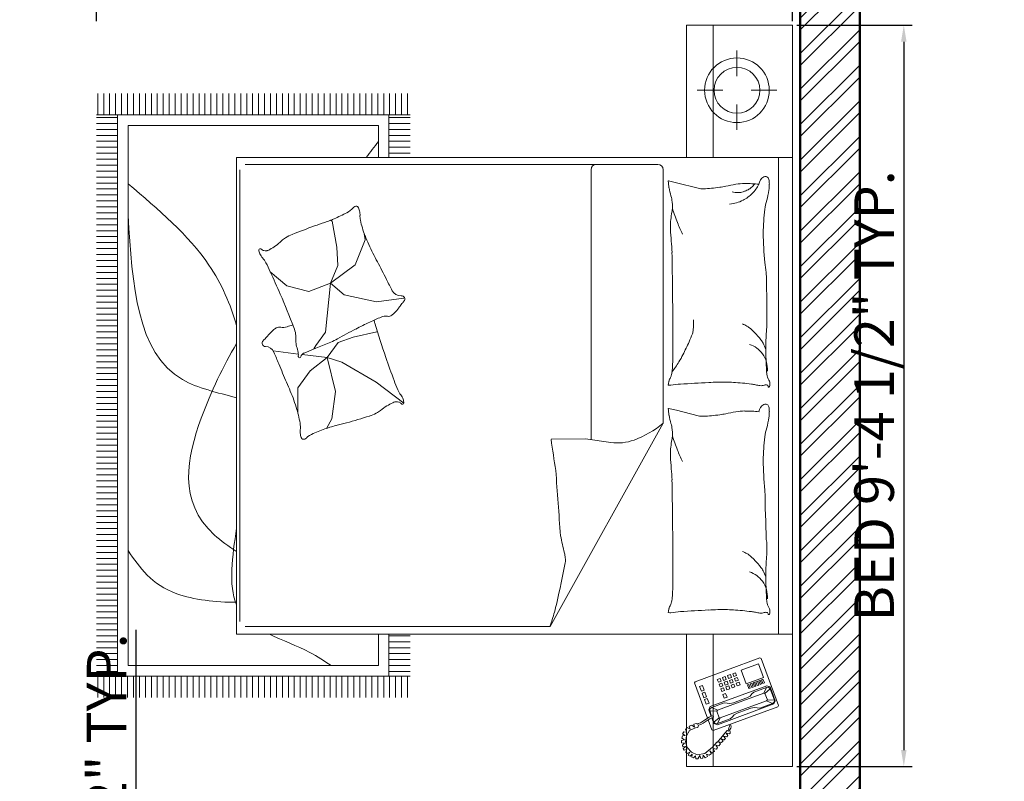
# Model space of a CAD drawing. Units: millimetres. Extents: x 20768 to 23556, y 50760 to 52704.
# Tile 22 of 36: x 21006 to 21155, y 52368 to 52483. Entities that reach past the tile are written whole.
import ezdxf

# ---------------------------------------------------------------- set-up
doc = ezdxf.new("R2010")
doc.units = ezdxf.units.MM
for name, color, linetype, lineweight in [('A-FURN', 8, 'Continuous', 18), ('A-WALL', 7, 'Continuous', 50), ('A-WALL-PATT', 8, 'Continuous', 13), ('S-ANNO-DIMS', 2, 'Continuous', 18)]:
    doc.layers.add(name, color=color, linetype=linetype, lineweight=lineweight)
doc.styles.add('DIM_FONT', font='SIMPLEX.shx', dxfattribs={"width": 0.8})
doc.styles.get("Standard").update_dxf_attribs({"font": 'arial.ttf'})
doc.dimstyles.new('ISO-25', dxfattribs={"dimtxt": 6, "dimasz": 2.5, "dimexe": 1.25, "dimexo": 0.625, "dimtad": 1, "dimdec": 0, "dimlunit": 3, "dimtxsty": 'Standard', "dimcen": 2.5, "dimadec": 0, "dimazin": 0, "dimtfac": 1, "dimtdec": 0, "dimtmove": 0, "dimatfit": 3, "dimfxl": 1, "dimarcsym": 0})

# ---------------------------------------------------------------- blocks, each defined once
blk = doc.blocks.new('A$C4F634EDD')
for p, q in [((0, 2.6295), (0, 2.2295)), ((0.5, 2.6295), (0, 2.6295)), ((0.5, 2.6295), (2.3, 2.6295)), ((0.5, 0.5295), (0.5, 2.6295)), ((0.5, 2.2295), (0.5, 2.6295)), ((2.3, 2.6295), (2.3, 0.5295)), ((2.3, 2.6295), (2.8, 2.6295)), ((2.3, 2.2295), (2.3, 2.6295)), ((2.8, 2.6295), (2.8, 2.2295)), ((0.2457, 2.5697), (0.2457, 2.4733)), ((0.5, 2.5771), (2.3, 2.5771)), ((2.392, 2.5115), (2.5692, 2.5765)), ((2.5692, 2.5765), (2.574, 2.5743)), ((2.574, 2.5743), (2.6638, 2.3298)), ((2.4946, 2.5331), (2.4985, 2.5445)), ((2.5734, 2.3187), (2.4946, 2.5331)), ((2.4985, 2.5445), (2.5516, 2.564)), ((2.5062, 2.5454), (2.5004, 2.5392)), ((2.5004, 2.5392), (2.5013, 2.5315)), ((2.5013, 2.5315), (2.5188, 2.4836)), ((2.5013, 2.5315), (2.5231, 2.5214)), ((2.5062, 2.5454), (2.5487, 2.561)), ((2.5235, 2.5256), (2.5062, 2.5454)), ((2.5483, 2.5347), (2.5235, 2.5256)), ((2.5483, 2.5347), (2.5487, 2.561)), ((2.5514, 2.5318), (2.5483, 2.5347)), ((2.5487, 2.561), (2.5571, 2.56)), ((2.5615, 2.5536), (2.5514, 2.5318)), ((2.5807, 2.4521), (2.5514, 2.5318)), ((2.5516, 2.564), (2.5637, 2.5584)), ((2.5571, 2.56), (2.5615, 2.5536)), ((2.5615, 2.5536), (2.5791, 2.5058)), ((2.5637, 2.5584), (2.6418, 2.3458)), ((2.3898, 2.5066), (2.392, 2.5115)), ((2.4795, 2.2621), (2.3898, 2.5066)), ((2.412, 2.5007), (2.4634, 2.5196)), ((2.4361, 2.4352), (2.412, 2.5007)), ((2.4634, 2.5196), (2.4875, 2.454)), ((2.4842, 2.5232), (2.47, 2.518)), ((2.47, 2.518), (2.472, 2.5127)), ((2.472, 2.5127), (2.4862, 2.5179)), ((2.4881, 2.5126), (2.4739, 2.5074)), ((2.4739, 2.5074), (2.4759, 2.502)), ((2.4759, 2.502), (2.4901, 2.5073)), ((2.492, 2.5019), (2.4778, 2.4967)), ((2.4778, 2.4967), (2.4798, 2.4914)), ((2.4798, 2.4914), (2.494, 2.4966)), ((2.4862, 2.5179), (2.4842, 2.5232)), ((2.4901, 2.5073), (2.4881, 2.5126)), ((2.494, 2.4966), (2.492, 2.5019)), ((2.5231, 2.5214), (2.5235, 2.5256)), ((2.5523, 2.4417), (2.5231, 2.5214)), ((2.5788, 2.4956), (2.5767, 2.4848)), ((2.5791, 2.5058), (2.5788, 2.4956)), ((2.4959, 2.4913), (2.4817, 2.4861)), ((2.4817, 2.4861), (2.4837, 2.4808)), ((2.4837, 2.4808), (2.4979, 2.486)), ((2.4998, 2.4807), (2.4856, 2.4755)), ((2.4856, 2.4755), (2.4876, 2.4702)), ((2.4876, 2.4702), (2.5018, 2.4754)), ((2.5037, 2.47), (2.4895, 2.4648)), ((2.4895, 2.4648), (2.4915, 2.4595)), ((2.4915, 2.4595), (2.5057, 2.4647)), ((2.4979, 2.486), (2.4959, 2.4913)), ((2.5018, 2.4754), (2.4998, 2.4807)), ((2.5057, 2.4647), (2.5037, 2.47)), ((2.5188, 2.4836), (2.5256, 2.4761)), ((2.5256, 2.4761), (2.5342, 2.4692)), ((2.5342, 2.4692), (2.5405, 2.4574)), ((2.5405, 2.4574), (2.547, 2.4397)), ((2.5767, 2.4848), (2.5795, 2.4717)), ((2.5795, 2.4717), (2.586, 2.454)), ((0.0957, 2.4197), (0.192, 2.4197)), ((0.2994, 2.4197), (0.3957, 2.4197)), ((2.4875, 2.454), (2.4361, 2.4352)), ((2.4457, 2.4146), (2.4563, 2.4185)), ((2.4563, 2.4185), (2.4602, 2.4078)), ((2.4634, 2.4211), (2.474, 2.425)), ((2.4673, 2.4104), (2.4634, 2.4211)), ((2.474, 2.425), (2.4779, 2.4143)), ((2.4811, 2.4276), (2.4917, 2.4315)), ((2.485, 2.4169), (2.4811, 2.4276)), ((2.4956, 2.4208), (2.485, 2.4169)), ((2.4917, 2.4315), (2.4956, 2.4208)), ((2.5594, 2.4061), (2.547, 2.4397)), ((2.5523, 2.4417), (2.5875, 2.346)), ((2.5807, 2.4521), (2.6158, 2.3564)), ((2.5984, 2.4204), (2.586, 2.454)), ((2.6047, 2.4086), (2.5984, 2.4204)), ((2.4496, 2.4039), (2.4457, 2.4146)), ((2.4602, 2.4078), (2.4496, 2.4039)), ((2.4528, 2.3951), (2.4635, 2.399)), ((2.4567, 2.3844), (2.4528, 2.3951)), ((2.4674, 2.3883), (2.4567, 2.3844)), ((2.4635, 2.399), (2.4674, 2.3883)), ((2.4779, 2.4143), (2.4673, 2.4104)), ((2.4706, 2.4016), (2.4812, 2.4055)), ((2.4745, 2.3909), (2.4706, 2.4016)), ((2.4851, 2.3949), (2.4745, 2.3909)), ((2.4777, 2.3821), (2.4883, 2.386)), ((2.4816, 2.3715), (2.4777, 2.3821)), ((2.4812, 2.4055), (2.4851, 2.3949)), ((2.4883, 2.4081), (2.4989, 2.412)), ((2.4922, 2.3975), (2.4883, 2.4081)), ((2.4883, 2.386), (2.4922, 2.3754)), ((2.5028, 2.4014), (2.4922, 2.3975)), ((2.4954, 2.3886), (2.5061, 2.3925)), ((2.4993, 2.378), (2.4954, 2.3886)), ((2.4989, 2.412), (2.5028, 2.4014)), ((2.51, 2.3819), (2.4993, 2.378)), ((2.5061, 2.3925), (2.51, 2.3819)), ((2.5238, 2.3769), (2.538, 2.3821)), ((2.538, 2.3821), (2.5419, 2.3715)), ((2.5622, 2.393), (2.5594, 2.4061)), ((2.5598, 2.372), (2.5601, 2.3822)), ((2.5601, 2.3822), (2.5622, 2.393)), ((2.6133, 2.4017), (2.6047, 2.4086)), ((2.6201, 2.3941), (2.6133, 2.4017)), ((2.6376, 2.3463), (2.6201, 2.3941)), ((2.6499, 2.3979), (2.6397, 2.3953)), ((2.6417, 2.39), (2.6488, 2.391)), ((2.6488, 2.391), (2.6538, 2.3895)), ((2.6551, 2.397), (2.6499, 2.3979)), ((2.6538, 2.3895), (2.6596, 2.388)), ((2.6627, 2.392), (2.6551, 2.397)), ((2.6596, 2.388), (2.6626, 2.3867)), ((2.6626, 2.3867), (2.6662, 2.388)), ((2.6692, 2.394), (2.6627, 2.392)), ((2.6662, 2.388), (2.6632, 2.3828)), ((2.6632, 2.3828), (2.6736, 2.3744)), ((2.6736, 2.3944), (2.6692, 2.394)), ((2.6765, 2.391), (2.6736, 2.3944)), ((2.6742, 2.3795), (2.6765, 2.391)), ((2.6824, 2.3858), (2.6742, 2.3795)), ((2.6873, 2.3815), (2.6824, 2.3858)), ((2.6853, 2.369), (2.6873, 2.3815)), ((0.2457, 2.366), (0.2457, 2.2697)), ((2.46, 2.3756), (2.4706, 2.3795)), ((2.4639, 2.365), (2.46, 2.3756)), ((2.4745, 2.3689), (2.4639, 2.365)), ((2.4672, 2.3561), (2.4778, 2.36)), ((2.4711, 2.3455), (2.4672, 2.3561)), ((2.4706, 2.3795), (2.4745, 2.3689)), ((2.4817, 2.3494), (2.4711, 2.3455)), ((2.4778, 2.36), (2.4817, 2.3494)), ((2.4922, 2.3754), (2.4816, 2.3715)), ((2.4849, 2.3626), (2.4955, 2.3665)), ((2.4888, 2.352), (2.4849, 2.3626)), ((2.4994, 2.3559), (2.4888, 2.352)), ((2.4955, 2.3665), (2.4994, 2.3559)), ((2.5026, 2.3691), (2.5132, 2.373)), ((2.5065, 2.3585), (2.5026, 2.3691)), ((2.5171, 2.3624), (2.5065, 2.3585)), ((2.5132, 2.373), (2.5171, 2.3624)), ((2.5277, 2.3663), (2.5238, 2.3769)), ((2.5419, 2.3715), (2.5277, 2.3663)), ((2.5774, 2.3242), (2.5598, 2.372)), ((2.5774, 2.3242), (2.5875, 2.346)), ((2.5875, 2.346), (2.5905, 2.3431)), ((2.5905, 2.3431), (2.5901, 2.3168)), ((2.6154, 2.3522), (2.5905, 2.3431)), ((2.6158, 2.3564), (2.6154, 2.3522)), ((2.6154, 2.3522), (2.6327, 2.3324)), ((2.6376, 2.3463), (2.6158, 2.3564)), ((2.6418, 2.3458), (2.6369, 2.332)), ((2.6385, 2.3386), (2.6376, 2.3463)), ((2.6736, 2.3744), (2.6922, 2.3593)), ((2.6946, 2.376), (2.6853, 2.369)), ((2.6922, 2.3593), (2.7051, 2.3473)), ((2.6995, 2.3713), (2.6946, 2.376)), ((2.695, 2.3603), (2.6995, 2.3713)), ((2.7031, 2.3682), (2.695, 2.3603)), ((2.7096, 2.3616), (2.7031, 2.3682)), ((2.7051, 2.3473), (2.7079, 2.3475)), ((2.7062, 2.351), (2.7096, 2.3616)), ((2.7147, 2.3578), (2.7062, 2.351)), ((2.7079, 2.3475), (2.7079, 2.3443)), ((2.7079, 2.3443), (2.727, 2.3277)), ((2.7214, 2.3517), (2.7147, 2.3578)), ((2.7196, 2.34), (2.7214, 2.3517)), ((2.7286, 2.3466), (2.7196, 2.34)), ((2.7346, 2.3423), (2.7286, 2.3466)), ((0, 2.3301), (0.5, 2.3301)), ((2.8, 2.3301), (2.3, 2.3301)), ((2.6172, 2.3086), (2.4844, 2.2599)), ((2.561, 2.3141), (2.5433, 2.3076)), ((2.5433, 2.3076), (2.5472, 2.297)), ((2.5649, 2.3035), (2.561, 2.3141)), ((2.5855, 2.3131), (2.5734, 2.3187)), ((2.5818, 2.3178), (2.5774, 2.3242)), ((2.5901, 2.3168), (2.5818, 2.3178)), ((2.6104, 2.3222), (2.5855, 2.3131)), ((2.5901, 2.3168), (2.6097, 2.324)), ((2.613, 2.3312), (2.6077, 2.3293)), ((2.6077, 2.3293), (2.6135, 2.3141)), ((2.6192, 2.3174), (2.613, 2.3312)), ((2.6135, 2.3141), (2.6244, 2.2977)), ((2.6153, 2.3261), (2.6327, 2.3324)), ((2.6369, 2.332), (2.6161, 2.3243)), ((2.626, 2.3069), (2.6192, 2.3174)), ((2.6616, 2.3249), (2.6234, 2.3109)), ((2.6365, 2.2916), (2.626, 2.3069)), ((2.6327, 2.3324), (2.6385, 2.3386)), ((2.6638, 2.3298), (2.6616, 2.3249)), ((2.727, 2.3277), (2.7512, 2.2983)), ((2.732, 2.3295), (2.7346, 2.3423)), ((2.7423, 2.3345), (2.732, 2.3295)), ((2.7406, 2.3172), (2.7495, 2.325)), ((2.7519, 2.3218), (2.7406, 2.3172)), ((2.7495, 2.325), (2.7423, 2.3345)), ((2.7575, 2.3144), (2.7519, 2.3218)), ((2.7526, 2.3045), (2.7575, 2.3144)), ((2.7622, 2.308), (2.7526, 2.3045)), ((2.7673, 2.2997), (2.7622, 2.308)), ((0.5953, 2.1912), (0.616, 2.2738)), ((1.4546, 2.1912), (1.4752, 2.2738)), ((2.5114, 2.2959), (2.4936, 2.2894)), ((2.4936, 2.2894), (2.4976, 2.2788)), ((2.4976, 2.2788), (2.5153, 2.2853)), ((2.5153, 2.2853), (2.5114, 2.2959)), ((2.5362, 2.305), (2.5185, 2.2985)), ((2.5185, 2.2985), (2.5224, 2.2879)), ((2.5224, 2.2879), (2.5401, 2.2944)), ((2.5401, 2.2944), (2.5362, 2.305)), ((2.5472, 2.297), (2.5649, 2.3035)), ((2.6244, 2.2977), (2.6349, 2.2825)), ((2.6349, 2.2825), (2.638, 2.273)), ((2.6407, 2.2834), (2.6365, 2.2916)), ((2.6399, 2.2712), (2.6374, 2.2659)), ((2.638, 2.273), (2.6399, 2.2712)), ((2.6438, 2.2739), (2.6407, 2.2834)), ((2.6519, 2.2716), (2.6438, 2.2739)), ((2.6535, 2.2628), (2.6519, 2.2716)), ((2.756, 2.2695), (2.7459, 2.2483)), ((2.7512, 2.2983), (2.756, 2.2695)), ((2.7574, 2.2924), (2.7673, 2.2997)), ((2.7687, 2.2905), (2.7574, 2.2924)), ((2.7587, 2.279), (2.7699, 2.2828)), ((2.7708, 2.2725), (2.7587, 2.279)), ((2.7699, 2.2828), (2.7687, 2.2905)), ((2.7706, 2.2643), (2.7708, 2.2725)), ((2.4844, 2.2599), (2.4795, 2.2621)), ((2.6374, 2.2659), (2.6398, 2.257)), ((2.6398, 2.257), (2.6509, 2.259)), ((2.6509, 2.259), (2.6431, 2.2492)), ((2.6431, 2.2492), (2.6473, 2.2398)), ((2.6473, 2.2398), (2.6592, 2.2429)), ((2.6592, 2.2429), (2.6521, 2.2314)), ((2.6636, 2.2409), (2.6535, 2.2628)), ((2.6836, 2.2287), (2.6636, 2.2409)), ((2.7284, 2.2317), (2.7063, 2.2256)), ((2.7459, 2.2483), (2.7284, 2.2317)), ((2.7509, 2.2314), (2.7459, 2.2418)), ((2.7459, 2.2418), (2.7568, 2.2352)), ((2.7529, 2.2505), (2.7645, 2.2498)), ((2.7607, 2.2424), (2.7529, 2.2505)), ((2.7568, 2.2352), (2.7607, 2.2424)), ((2.759, 2.2637), (2.7706, 2.2643)), ((2.7676, 2.2559), (2.759, 2.2637)), ((2.7645, 2.2498), (2.7676, 2.2559)), ((0, 2.2295), (0.5, 2.2295)), ((2.8, 2.2295), (2.3, 2.2295)), ((2.6521, 2.2314), (2.6598, 2.2248)), ((2.6598, 2.2248), (2.6697, 2.2309)), ((2.6697, 2.2309), (2.6684, 2.219)), ((2.6684, 2.219), (2.6761, 2.2145)), ((2.6761, 2.2145), (2.6821, 2.2237)), ((2.6821, 2.2237), (2.6843, 2.2135)), ((2.7063, 2.2256), (2.6836, 2.2287)), ((2.6843, 2.2135), (2.6927, 2.2117)), ((2.6927, 2.2117), (2.6986, 2.222)), ((2.6986, 2.222), (2.7019, 2.2098)), ((2.7019, 2.2098), (2.7102, 2.2104)), ((2.7102, 2.2104), (2.7113, 2.2218)), ((2.7113, 2.2218), (2.7192, 2.2137)), ((2.7192, 2.2137), (2.7255, 2.2152)), ((2.7255, 2.2152), (2.7242, 2.2265)), ((2.7242, 2.2265), (2.7324, 2.2165)), ((2.7324, 2.2165), (2.7386, 2.2208)), ((2.7386, 2.2208), (2.7354, 2.2306)), ((2.7354, 2.2306), (2.7462, 2.2264)), ((2.7462, 2.2264), (2.7509, 2.2314)), ((0.5878, 2.1612), (0.5953, 2.1912)), ((1.4471, 2.1612), (1.4546, 2.1912)), ((0.5258, 2.121), (0.5258, 0.5617)), ((1.5035, 2.141), (0.5458, 2.141)), ((1.5035, 2.141), (2.2716, 1.7136)), ((1.576, 1.9433), (1.5624, 1.8479)), ((0.5458, 1.8684), (1.5653, 1.8684)), ((1.5624, 1.8479), (1.5641, 1.7178)), ((2.2716, 0.5617), (2.2716, 1.7136)), ((0.2586, 1.1753), (0.3386, 1.1753)), ((0.3386, 0), (0.3386, 1.1852)), ((0.3486, 1.1052), (0.3486, 1.1852)), ((0.3711, 1.1052), (0.3711, 1.1852)), ((0.3936, 1.1052), (0.3936, 1.1852)), ((0.4161, 1.1052), (0.4161, 1.1852)), ((0.4386, 1.1052), (0.4386, 1.1852)), ((0.4611, 1.1052), (0.4611, 1.1852)), ((0.4836, 1.1052), (0.4836, 1.1852)), ((1.031, 1.1612), (1.0448, 1.0581)), ((1.4276, 1.1611), (1.3484, 1.0571)), ((2.3061, 1.1052), (2.3061, 1.1852)), ((2.3286, 1.1052), (2.3286, 1.1852)), ((2.3511, 1.1052), (2.3511, 1.1852)), ((2.3736, 1.1052), (2.3736, 1.1852)), ((2.3961, 1.1052), (2.3961, 1.1852)), ((2.4186, 1.1052), (2.4186, 1.1852)), ((2.4411, 1.1052), (2.4411, 1.1852)), ((2.4588, 1.1852), (2.4588, 0)), ((2.4588, 1.1753), (2.5388, 1.1753)), ((0.2586, 1.1528), (0.3386, 1.1528)), ((0.2586, 1.1303), (0.3386, 1.1303)), ((2.4588, 1.1528), (2.5388, 1.1528)), ((2.4588, 1.1303), (2.5388, 1.1303)), ((0.2586, 1.1078), (0.3386, 1.1078)), ((0.2586, 1.0853), (0.3386, 1.0853)), ((0.3386, 1.1052), (0.5, 1.1052)), ((2.3, 1.1052), (2.4588, 1.1052)), ((2.4588, 1.1078), (2.5388, 1.1078)), ((2.4588, 1.0853), (2.5388, 1.0853)), ((0.2586, 1.0628), (0.3386, 1.0628)), ((0.3786, 1.0652), (0.5, 1.0652)), ((0.3786, 0.12), (0.3786, 1.0652)), ((1.0448, 1.0581), (1.019, 0.936)), ((1.1784, 0.9702), (1.1586, 1.0591)), ((1.3484, 1.0571), (1.2733, 0.9268)), ((2.3, 1.0652), (2.4188, 1.0652)), ((2.4188, 1.0652), (2.4188, 0.12)), ((2.4588, 1.0628), (2.5388, 1.0628)), ((0.2586, 1.0403), (0.3386, 1.0403)), ((0.2586, 1.0178), (0.3386, 1.0178)), ((0.8108, 1.0151), (0.7868, 1.0117)), ((0.9054, 0.9773), (0.8108, 1.0151)), ((2.4588, 1.0403), (2.5388, 1.0403)), ((2.4588, 1.0178), (2.5388, 1.0178)), ((0.2586, 0.9953), (0.3386, 0.9953)), ((0.2586, 0.9728), (0.3386, 0.9728)), ((0.9743, 0.8845), (0.9054, 0.9773)), ((1.1982, 0.9129), (1.1784, 0.9702)), ((2.4588, 0.9953), (2.5388, 0.9953)), ((2.4588, 0.9728), (2.5388, 0.9728)), ((0.2586, 0.9503), (0.3386, 0.9503)), ((1.019, 0.936), (0.9743, 0.8845)), ((2.4588, 0.9503), (2.5388, 0.9503)), ((0.2586, 0.9278), (0.3386, 0.9278)), ((0.2586, 0.9053), (0.3386, 0.9053)), ((0.8384, 0.9085), (0.7403, 0.8913)), ((0.9072, 0.912), (0.8384, 0.9085)), ((0.9743, 0.8845), (0.9072, 0.912)), ((1.2555, 0.8715), (1.1982, 0.9129)), ((1.2733, 0.9268), (1.2555, 0.8715)), ((1.2555, 0.8715), (1.384, 0.9031)), ((1.384, 0.9031), (1.4868, 0.8892)), ((2.4588, 0.9278), (2.5388, 0.9278)), ((2.4588, 0.9053), (2.5388, 0.9053)), ((0.2586, 0.8828), (0.3386, 0.8828)), ((0.2586, 0.8603), (0.3386, 0.8603)), ((0.7403, 0.8913), (0.737, 0.8849)), ((0.9743, 0.8845), (1.0052, 0.802)), ((0.9743, 0.8845), (1.16, 0.8656)), ((1.16, 0.8656), (1.2099, 0.8295)), ((1.1973, 0.8853), (1.2203, 0.829)), ((1.2555, 0.8715), (1.2437, 0.7773)), ((1.2555, 0.8715), (1.3049, 0.8082)), ((1.4868, 0.8892), (1.5228, 0.8692)), ((2.4588, 0.8828), (2.5388, 0.8828)), ((2.4588, 0.8603), (2.5388, 0.8603)), ((0.2586, 0.8378), (0.3386, 0.8378)), ((1.2099, 0.8295), (1.222, 0.8209)), ((1.2203, 0.829), (1.2381, 0.7855)), ((2.4588, 0.8378), (2.5388, 0.8378)), ((0.2586, 0.8153), (0.3386, 0.8153)), ((0.2586, 0.7928), (0.3386, 0.7928)), ((1.0052, 0.802), (0.9846, 0.7194)), ((1.3049, 0.8082), (1.3701, 0.7608)), ((2.4588, 0.8153), (2.5388, 0.8153)), ((2.4588, 0.7928), (2.5388, 0.7928)), ((0.2586, 0.7703), (0.3386, 0.7703)), ((0.2586, 0.7478), (0.3386, 0.7478)), ((1.2419, 0.7626), (1.23, 0.668)), ((1.3701, 0.7608), (1.463, 0.7608)), ((2.4588, 0.7703), (2.5388, 0.7703)), ((2.4588, 0.7478), (2.5388, 0.7478)), ((0.2586, 0.7253), (0.3386, 0.7253)), ((0.9846, 0.7194), (0.931, 0.6569)), ((2.4588, 0.7253), (2.5388, 0.7253)), ((0.2586, 0.7028), (0.3386, 0.7028)), ((0.2586, 0.6803), (0.3386, 0.6803)), ((2.4588, 0.7028), (2.5388, 0.7028)), ((2.4588, 0.6803), (2.5388, 0.6803)), ((0.2586, 0.6578), (0.3386, 0.6578)), ((0.2586, 0.6353), (0.3386, 0.6353)), ((2.4588, 0.6578), (2.5388, 0.6578)), ((2.4588, 0.6353), (2.5388, 0.6353)), ((0.2586, 0.6128), (0.3386, 0.6128)), ((2.4588, 0.6128), (2.5388, 0.6128)), ((0.2586, 0.5903), (0.3386, 0.5903)), ((0.2586, 0.5678), (0.3386, 0.5678)), ((2.4588, 0.5903), (2.5388, 0.5903)), ((2.4588, 0.5678), (2.5388, 0.5678)), ((0.2586, 0.5453), (0.3386, 0.5453)), ((0.2586, 0.5228), (0.3386, 0.5228)), ((2.3, 0.5295), (0.5, 0.5295)), ((0.5458, 0.5417), (2.2516, 0.5417)), ((2.4588, 0.5453), (2.5388, 0.5453)), ((2.4588, 0.5228), (2.5388, 0.5228)), ((0.2586, 0.5003), (0.3386, 0.5003)), ((2.4588, 0.5003), (2.5388, 0.5003)), ((0.2586, 0.4778), (0.3386, 0.4778)), ((0.2586, 0.4553), (0.3386, 0.4553)), ((2.4588, 0.4778), (2.5388, 0.4778)), ((2.4588, 0.4553), (2.5388, 0.4553)), ((0.2586, 0.4328), (0.3386, 0.4328)), ((0.2586, 0.4103), (0.3386, 0.4103)), ((2.4588, 0.4328), (2.5388, 0.4328)), ((2.4588, 0.4103), (2.5388, 0.4103)), ((0.2586, 0.3878), (0.3386, 0.3878)), ((2.4588, 0.3878), (2.5388, 0.3878)), ((0.2586, 0.3653), (0.3386, 0.3653)), ((0.2586, 0.3428), (0.3386, 0.3428)), ((2.4588, 0.3653), (2.5388, 0.3653)), ((2.4588, 0.3428), (2.5388, 0.3428)), ((0.2586, 0.3203), (0.3386, 0.3203)), ((0.2586, 0.2978), (0.3386, 0.2978)), ((2.4588, 0.3203), (2.5388, 0.3203)), ((2.4588, 0.2978), (2.5388, 0.2978)), ((0.2586, 0.2753), (0.3386, 0.2753)), ((2.4588, 0.2753), (2.5388, 0.2753)), ((0.2586, 0.2528), (0.3386, 0.2528)), ((0.2586, 0.2303), (0.3386, 0.2303)), ((2.4588, 0.2528), (2.5388, 0.2528)), ((2.4588, 0.2303), (2.5388, 0.2303)), ((0.2586, 0.2078), (0.3386, 0.2078)), ((2.4588, 0.2078), (2.5388, 0.2078)), ((0.2586, 0.1853), (0.3386, 0.1853)), ((0.2586, 0.1628), (0.3386, 0.1628)), ((2.4588, 0.1853), (2.5388, 0.1853)), ((2.4588, 0.1628), (2.5388, 0.1628)), ((0.2586, 0.1403), (0.3386, 0.1403)), ((0.2586, 0.1178), (0.3386, 0.1178)), ((2.4188, 0.12), (0.3786, 0.12)), ((2.4588, 0.1403), (2.5388, 0.1403)), ((2.4588, 0.1178), (2.5388, 0.1178)), ((0.2586, 0.0953), (0.3386, 0.0953)), ((2.4588, 0.08), (0.3386, 0.08)), ((0.3486, 0), (0.3486, 0.08)), ((0.3711, 0), (0.3711, 0.08)), ((0.3936, 0), (0.3936, 0.08)), ((0.4161, 0), (0.4161, 0.08)), ((0.4386, 0), (0.4386, 0.08)), ((0.4611, 0), (0.4611, 0.08)), ((0.4836, 0), (0.4836, 0.08)), ((0.5061, 0), (0.5061, 0.08)), ((0.5286, 0), (0.5286, 0.08)), ((0.5511, 0), (0.5511, 0.08)), ((0.5736, 0), (0.5736, 0.08)), ((0.5961, 0), (0.5961, 0.08)), ((0.6186, 0), (0.6186, 0.08)), ((0.6411, 0), (0.6411, 0.08)), ((0.6636, 0), (0.6636, 0.08)), ((0.6861, 0), (0.6861, 0.08)), ((0.7086, 0), (0.7086, 0.08)), ((0.7311, 0), (0.7311, 0.08)), ((0.7536, 0), (0.7536, 0.08)), ((0.7761, 0), (0.7761, 0.08)), ((0.7986, 0), (0.7986, 0.08)), ((0.8211, 0), (0.8211, 0.08)), ((0.8436, 0), (0.8436, 0.08)), ((0.8661, 0), (0.8661, 0.08)), ((0.8886, 0), (0.8886, 0.08)), ((0.9111, 0), (0.9111, 0.08)), ((0.9336, 0), (0.9336, 0.08)), ((0.9561, 0), (0.9561, 0.08)), ((0.9786, 0), (0.9786, 0.08)), ((1.0011, 0), (1.0011, 0.08)), ((1.0236, 0), (1.0236, 0.08)), ((1.0461, 0), (1.0461, 0.08)), ((1.0686, 0), (1.0686, 0.08)), ((1.0911, 0), (1.0911, 0.08)), ((1.1136, 0), (1.1136, 0.08)), ((1.1361, 0), (1.1361, 0.08)), ((1.1586, 0), (1.1586, 0.08)), ((1.1811, 0), (1.1811, 0.08)), ((1.2036, 0), (1.2036, 0.08)), ((1.2261, 0), (1.2261, 0.08)), ((1.2486, 0), (1.2486, 0.08)), ((1.2711, 0), (1.2711, 0.08)), ((1.2936, 0), (1.2936, 0.08)), ((1.3161, 0), (1.3161, 0.08)), ((1.3386, 0), (1.3386, 0.08)), ((1.3611, 0), (1.3611, 0.08)), ((1.3836, 0), (1.3836, 0.08)), ((1.4061, 0), (1.4061, 0.08)), ((1.4286, 0), (1.4286, 0.08)), ((1.4511, 0), (1.4511, 0.08)), ((1.4736, 0), (1.4736, 0.08)), ((1.4961, 0), (1.4961, 0.08)), ((1.5186, 0), (1.5186, 0.08)), ((1.5411, 0), (1.5411, 0.08)), ((1.5636, 0), (1.5636, 0.08)), ((1.5861, 0), (1.5861, 0.08)), ((1.6086, 0), (1.6086, 0.08)), ((1.6311, 0), (1.6311, 0.08)), ((1.6536, 0), (1.6536, 0.08)), ((1.6761, 0), (1.6761, 0.08)), ((1.6986, 0), (1.6986, 0.08)), ((1.7211, 0), (1.7211, 0.08)), ((1.7436, 0), (1.7436, 0.08)), ((1.7661, 0), (1.7661, 0.08)), ((1.7886, 0), (1.7886, 0.08)), ((1.8111, 0), (1.8111, 0.08)), ((1.8336, 0), (1.8336, 0.08)), ((1.8561, 0), (1.8561, 0.08)), ((1.8786, 0), (1.8786, 0.08)), ((1.9011, 0), (1.9011, 0.08)), ((1.9236, 0), (1.9236, 0.08)), ((1.9461, 0), (1.9461, 0.08)), ((1.9686, 0), (1.9686, 0.08)), ((1.9911, 0), (1.9911, 0.08)), ((2.0136, 0), (2.0136, 0.08)), ((2.0361, 0), (2.0361, 0.08)), ((2.0586, 0), (2.0586, 0.08)), ((2.0811, 0), (2.0811, 0.08)), ((2.1036, 0), (2.1036, 0.08)), ((2.1261, 0), (2.1261, 0.08)), ((2.1486, 0), (2.1486, 0.08)), ((2.1711, 0), (2.1711, 0.08)), ((2.1936, 0), (2.1936, 0.08)), ((2.2161, 0), (2.2161, 0.08)), ((2.2386, 0), (2.2386, 0.08)), ((2.2611, 0), (2.2611, 0.08)), ((2.2836, 0), (2.2836, 0.08)), ((2.3061, 0), (2.3061, 0.08)), ((2.3286, 0), (2.3286, 0.08)), ((2.3511, 0), (2.3511, 0.08)), ((2.3736, 0), (2.3736, 0.08)), ((2.3961, 0), (2.3961, 0.08)), ((2.4186, 0), (2.4186, 0.08)), ((2.4411, 0), (2.4411, 0.08)), ((2.4588, 0.0953), (2.5388, 0.0953)), ((0.2586, 0.0728), (0.3386, 0.0728)), ((0.2586, 0.0503), (0.3386, 0.0503)), ((2.4588, 0.0728), (2.5388, 0.0728)), ((2.4588, 0.0503), (2.5388, 0.0503)), ((0.2586, 0.0278), (0.3386, 0.0278)), ((0.2586, 0.0053), (0.3386, 0.0053)), ((2.4588, 0.0278), (2.5388, 0.0278)), ((2.4588, 0.0053), (2.5388, 0.0053))]:
    blk.add_line(p, q)
for radius in [0.1222, 0.0865]:
    blk.add_circle((0.2457, 2.4197), radius)
for centre, radius, start, end in [((0.5848, 2.5274), 0.0131, 101.2724, 206.5805), ((0.5999, 2.4516), 0.0904, 90, 101.2724), ((0.5999, 2.3808), 0.1611, 81.5628, 90), ((0.5788, 2.2388), 0.3048, 74.256, 81.5628), ((0.7272, 2.7653), 0.2422, 254.256, 262.4531), ((0.8402, 3.0514), 0.5293, 276.0867, 280.1899), ((1.1602, -8.1346), 10.6675, 90.30153, 91.21582), ((1.1169, 2.2433), 0.2897, 85.1982, 92.5386), ((1.2142, 3.4021), 0.8732, 265.1982, 269.4243), ((1.2204, 4.0232), 1.4943, 269.4243, 271.9079), ((1.2995, 2.4357), 0.0992, 105.9352, 126.0864), ((1.2429, 3.3501), 0.8208, 271.9079, 275.2592), ((1.2995, 2.4357), 0.0992, 85.7841, 105.9352), ((1.3132, 2.5864), 0.0539, 275.2592, 300.6513), ((1.3554, 2.5152), 0.0289, 85.6975, 120.6513), ((1.3556, 2.519), 0.0251, 68.2117, 85.6975), ((1.3739, 2.5288), 0.0156, 158.0096, 201.421), ((1.3634, 2.533), 0.00428, 78.1069, 158.0096), ((1.3647, 2.5395), 0.00232, 258.1069, 19.564), ((1.3637, 2.5391), 0.00342, 19.564, 68.2117), ((1.444, 2.5274), 0.0131, 101.2724, 206.5805), ((1.4591, 2.4516), 0.0904, 90, 101.2724), ((1.4591, 2.3808), 0.1611, 81.5628, 90), ((1.438, 2.2388), 0.3048, 74.256, 81.5628), ((1.5865, 2.7653), 0.2422, 254.256, 262.4531), ((1.4785, 15.4878), 12.9656, 271.22425, 272.05324), ((1.97, 2.3805), 0.1524, 92.5386, 100.1899), ((1.9761, 2.2433), 0.2897, 85.1982, 92.5386), ((2.0734, 3.4021), 0.8732, 265.1982, 269.4243), ((2.0797, 4.0232), 1.4943, 269.4243, 271.9079), ((2.1588, 2.4357), 0.0992, 105.9352, 126.0864), ((2.1021, 3.3501), 0.8208, 271.9079, 275.2592), ((2.1588, 2.4357), 0.0992, 85.7841, 105.9352), ((2.1724, 2.5864), 0.0539, 275.2592, 300.6513), ((2.2146, 2.5152), 0.0289, 85.6975, 120.6513), ((2.2149, 2.519), 0.0251, 68.2117, 85.6975), ((2.2331, 2.5288), 0.0156, 158.0096, 201.421), ((2.2226, 2.533), 0.00428, 78.1069, 158.0096), ((2.224, 2.5395), 0.00232, 258.1069, 19.564), ((2.2229, 2.5391), 0.00342, 19.564, 68.2117), ((0.6036, 2.5368), 0.0342, 206.5805, 265.5998), ((1.0898, 2.4496), 0.4918, 173.7676, 180), ((0.5368, 2.3783), 0.1399, 45.0976, 62.7964), ((0.7851, 3.2019), 0.6827, 262.4531, 270), ((0.7851, 3.5682), 1.049, 270, 276.0867), ((1.4317, 2.2032), 0.3916, 128.3886, 133.8115), ((1.2362, 2.45), 0.0768, 117.2396, 128.3886), ((1.3082, 2.3102), 0.234, 110.8603, 117.2396), ((1.2995, 2.4357), 0.0992, 143.8234, 161.5603), ((1.2995, 2.4357), 0.0992, 126.0864, 143.8234), ((1.1177, 2.5413), 0.246, 347.8905, 351.8665), ((1.3288, 2.5111), 0.0328, 351.8665, 21.421), ((1.4628, 2.5368), 0.0342, 206.5805, 265.5998), ((1.949, 2.4496), 0.4918, 173.7676, 180), ((1.6443, 3.2019), 0.6827, 262.4531, 270), ((1.6443, 3.5682), 1.049, 270, 276.0867), ((2.291, 2.2032), 0.3916, 128.3886, 133.8115), ((2.0954, 2.45), 0.0768, 117.2396, 128.3886), ((2.1674, 2.3102), 0.234, 110.8603, 117.2396), ((2.1588, 2.4357), 0.0992, 143.8234, 161.5603), ((2.1588, 2.4357), 0.0992, 126.0864, 143.8234), ((1.977, 2.5413), 0.246, 347.8905, 351.8665), ((2.1881, 2.5111), 0.0328, 351.8665, 21.421), ((0.5462, 2.4142), 0.0899, 41.4429, 53.7359), ((0.5741, 2.4389), 0.0526, 25.3551, 41.4429), ((0.4851, 2.3967), 0.1511, 21.8149, 25.3551), ((0.5368, 2.3783), 0.1399, 27.3988, 45.0976), ((1.3127, 2.3625), 0.2002, 151.6832, 156.9972), ((1.1799, 2.4341), 0.0493, 140.9651, 151.6832), ((1.3165, 2.3233), 0.2252, 133.8115, 140.9651), ((2.2605, 2.3525), 0.9131, 172.3191, 176.6313), ((1.5522, 2.448), 0.1983, 167.8905, 172.3191), ((2.1719, 2.3625), 0.2002, 151.6832, 156.9972), ((2.0391, 2.4341), 0.0493, 140.9651, 151.6832), ((2.1757, 2.3233), 0.2252, 133.8115, 140.9651), ((3.1198, 2.3525), 0.9131, 172.3191, 176.6313), ((2.4114, 2.448), 0.1983, 167.8905, 172.3191), ((0.8019, 2.4496), 0.204, 180, 189.6844), ((0.4345, 2.3765), 0.2056, 18.7799, 21.8149), ((0.576, 2.4246), 0.0562, 0, 18.7799), ((0.5406, 2.4246), 0.0915, 345.3149, 0), ((0.5368, 2.3783), 0.1399, 16.515, 27.3988), ((0.5368, 2.3783), 0.1399, 5.6311, 16.515), ((1.6611, 2.4496), 0.204, 180, 189.6844), ((1.4703, 2.5637), 0.882, 189.6844, 192.1984), ((2.0266, 2.3663), 0.6787, 176.6313, 181.6331), ((2.3295, 2.5637), 0.882, 189.6844, 192.1984), ((2.8858, 2.3663), 0.6787, 176.6313, 181.6331), ((0.2982, 2.3103), 0.3171, 8.0051, 12.1984), ((-0.0401, 2.2627), 0.6588, 2.6649, 8.0051), ((2.7128, 2.3859), 1.3652, 181.6331, 183.055), ((1.1575, 2.3103), 0.3171, 8.0051, 12.1984), ((0.8191, 2.2627), 0.6588, 2.6649, 8.0051), ((3.5721, 2.3859), 1.3652, 181.6331, 183.055), ((14.9657, 3.0398), 13.6356, 183.05496, 183.50486), ((15.8249, 3.0398), 13.6356, 183.05496, 183.50486), ((0.5503, 2.2902), 0.0677, 345.9548, 2.6649), ((1.4096, 2.2902), 0.0677, 345.9548, 2.6649), ((1.1303, 1.9835), 0.2721, 85.9172, 93.5552), ((1.1455, 2.197), 0.058, 69.3257, 85.9172), ((0.9871, 1.7772), 0.5066, 65.6735, 69.3257), ((0.6058, 0.9338), 1.4323, 63.5015, 65.6735), ((0.473, 2.8815), 0.7387, 289.428, 291.6577), ((0.473, 2.8815), 0.7387, 291.6577, 293.4844), ((0.473, 2.8815), 0.7387, 293.4844, 295.3111), ((1.1054, 1.9358), 0.3126, 57.865, 63.5015), ((0.8841, 1.5835), 0.7286, 54.1737, 57.865), ((1.6762, 2.2258), 0.3212, 183.5049, 189.9984), ((1.3322, 2.8815), 0.7387, 289.428, 291.6577), ((1.3322, 2.8815), 0.7387, 291.6577, 293.4844), ((1.3322, 2.8815), 0.7387, 293.4844, 295.3111), ((2.5355, 2.2258), 0.3212, 183.5049, 189.9984), ((0.5887, 2.1609), 0.000917, 165.9551, 274.0829), ((0.5695, 2.4301), 0.2708, 274.0829, 279.4841), ((0.5763, 2.3896), 0.2297, 279.4841, 287.3864), ((0.6807, 2.0561), 0.1197, 96.4341, 107.3864), ((0.6836, 2.0301), 0.1459, 78.4414, 96.4341), ((0.473, 2.8815), 0.7387, 287.1982, 289.428), ((0.759, 2.3985), 0.2301, 258.4414, 272.7491), ((0.7026, 3.5718), 1.4048, 272.7491, 274.6176), ((0.9136, 0.9591), 1.2165, 92.6096, 94.6176), ((1.2501, -19.8405), 22.0183, 90.37908, 91.01965), ((1.2012, -3.5404), 5.7185, 89.7135, 90.9704), ((1.224, 1.0141), 1.164, 86.426, 89.7135), ((1.2875, 2.0302), 0.1459, 77.131, 86.426), ((1.3099, 2.1283), 0.0453, 62.7159, 77.131), ((1.3658, 2.2367), 0.0767, 242.7159, 253.7788), ((1.3688, 2.247), 0.0875, 253.7788, 262.8796), ((1.3581, 2.1615), 0.00132, 262.8796, 343.3022), ((1.3409, 2.1667), 0.0193, 343.3022, 9.9984), ((1.448, 2.1609), 0.000917, 165.9551, 274.0829), ((1.4288, 2.4301), 0.2708, 274.0829, 279.4841), ((1.4355, 2.3896), 0.2297, 279.4841, 287.3864), ((1.5399, 2.0561), 0.1197, 96.4341, 107.3864), ((1.5429, 2.0301), 0.1459, 78.4414, 96.4341), ((1.3322, 2.8815), 0.7387, 287.1982, 289.428), ((1.6182, 2.3985), 0.2301, 258.4414, 272.7491), ((1.5619, 3.5718), 1.4048, 272.7491, 274.6176), ((1.7729, 0.9591), 1.2165, 92.6096, 94.6176), ((2.1093, -19.8405), 22.0183, 90.37908, 91.01965), ((2.0605, -3.5404), 5.7185, 89.7135, 90.9704), ((2.0833, 1.0141), 1.164, 86.426, 89.7135), ((2.1467, 2.0302), 0.1459, 77.131, 86.426), ((2.1691, 2.1283), 0.0453, 62.7159, 77.131), ((2.2251, 2.2367), 0.0767, 242.7159, 253.7788), ((2.2281, 2.247), 0.0875, 253.7788, 262.8796), ((2.2174, 2.1615), 0.00132, 262.8796, 343.3022), ((2.2001, 2.1667), 0.0193, 343.3022, 9.9984), ((0.5458, 2.121), 0.02, 90, 180), ((1.2147, 1.9017), 0.3751, 20.1488, 39.6445), ((1.3977, 1.9688), 0.1801, 351.8644, 20.1488), ((0.5458, 1.8884), 0.02, 180, 270), ((0.6102, 18.0525), 16.3521, 273.75703, 274.62393), ((1.4194, 4.2174), 2.5158, 281.6741, 283.1904), ((2.0378, 1.5789), 0.1942, 97.7304, 103.1904), ((2.0195, 1.7137), 0.0581, 79.2724, 97.7304), ((1.2737, -2.2227), 4.0646, 77.0745, 79.2724), ((1.0582, 5.4638), 3.7801, 277.692, 279.495), ((2.0359, 1.0981), 0.6574, 74.0648, 77.0745), ((1.7125, -0.0344), 1.8351, 72.2636, 74.0648), ((1.0348, 1.1521), 0.0127, 51.1864, 183.2455), ((0.9991, 1.1077), 0.0697, 45.8726, 51.1864), ((1.0791, 1.1902), 0.0452, 225.8726, 232.4713), ((1.2846, 1.4577), 0.3825, 232.4713, 233.7837), ((1.4338, 1.1026), 0.0601, 110.3452, 128.5854), ((1.4251, 1.1259), 0.0352, 86.0516, 110.3452), ((1.4273, 1.1567), 0.00443, 13.2808, 86.0516), ((1.4254, 1.1562), 0.0063, 306.5792, 13.2808), ((-0.4173, 3.8699), 3.0972, 296.4147, 297.2902), ((0.9863, 1.1494), 0.0359, 297.2902, 3.2455), ((0.6683, 0.6162), 0.6605, 52.7849, 53.7837), ((0.9362, 0.9689), 0.2176, 46.4776, 52.7849), ((1.0327, 1.0706), 0.0774, 35.8936, 46.4776), ((1.0771, 1.1027), 0.0226, 351.9508, 35.8936), ((-0.4107, 5.9078), 5.0942, 289.0836, 290.1287), ((1.0543, 1.9106), 0.8371, 290.1287, 292.7069), ((1.3469, 1.2115), 0.0792, 292.7069, 308.5854), ((1.4996, 1.1284), 0.0771, 169.5926, 177.2714), ((1.4378, 1.1314), 0.0153, 177.2714, 194.5709), ((1.4611, 1.1374), 0.0393, 194.5709, 206.8179), ((1.4376, 1.1398), 0.0142, 126.5792, 169.5926), ((1.7401, 1.2785), 0.352, 206.8179, 210.9056), ((3.744, -4.3336), 6.1019, 117.49986, 117.84822), ((1.8575, -0.7096), 2.0162, 116.4147, 117.4999), ((1.1449, 1.0931), 0.0458, 171.9508, 202.4162), ((0.2266, 4.0657), 3.145, 286.6085, 289.0836), ((1.6045, 1.1973), 0.194, 210.9056, 219.7005), ((0.5736, 1.5979), 0.6236, 290.7486, 297.4921), ((-1.8336, 6.2238), 5.8383, 297.49208, 297.84822), ((2.032, 1.4591), 1.0054, 202.4162, 205.0529), ((1.0922, 1.1636), 0.1166, 280.7366, 286.6085), ((1.3929, 1.0217), 0.081, 26.0735, 39.7005), ((1.2892, 0.9709), 0.1965, 17.8396, 26.0735), ((0.6422, 1.4168), 0.43, 282.6252, 290.7486), ((2.6493, 1.7476), 1.6868, 205.0529, 207.0884), ((-0.4304, 0.4175), 2.003, 15.2625, 17.8396), ((0.6894, 0.9832), 0.0058, 121.6917, 179.0386), ((0.7004, 0.983), 0.0168, 179.0386, 229.4914), ((0.7131, 0.9448), 0.0509, 103.0402, 121.6917), ((0.6405, 0.9128), 0.0755, 26.3332, 49.4914), ((0.7152, 0.9361), 0.0599, 86.6119, 103.0402), ((0.7224, 1.0587), 0.063, 266.6119, 282.6252), ((2.541, 1.6922), 1.5652, 207.0884, 209.936), ((-1.6775, -0.2344), 2.6619, 25.1732, 26.3332), ((-0.0881, 0.5109), 1.6481, 13.841, 15.2625), ((0.5689, 0.8213), 0.1798, 20.7081, 25.1732), ((0.9989, 0.8042), 0.2143, 22.2355, 29.936), ((2.0418, 1.0357), 0.5454, 193.841, 196.3122), ((0.2268, 0.692), 0.5454, 18.2369, 20.7081), ((2.3102, 1.3785), 1.6481, 198.2369, 199.6584), ((1.6908, 0.933), 0.1798, 196.3122, 200.7773), ((4.0115, 1.8135), 2.6619, 200.7773, 201.9373), ((2.6444, 1.4979), 2.003, 199.6584, 202.2355), ((1.6124, 0.8472), 0.0755, 201.9373, 225.0955), ((1.2594, 0.7942), 0.0231, 202.2355, 252.8133), ((1.5473, 0.7819), 0.0168, 354.6428, 45.0955), ((2.2689, -2.1899), 3.145, 111.0043, 113.4795), ((1.1834, 0.6373), 0.1166, 98.1216, 111.0043), ((1.1763, 0.687), 0.0663, 85.4882, 98.1216), ((1.1871, 0.8241), 0.0712, 265.4882, 277.6784), ((1.1727, 0.9313), 0.1794, 277.6784, 284.8807), ((1.2689, 0.569), 0.1955, 97.9822, 104.8807), ((1.2465, 0.729), 0.034, 85.7407, 97.9822), ((1.2497, 0.772), 0.0092, 265.7407, 289.3799), ((1.2512, 0.7678), 0.00467, 289.3799, 72.8133), ((1.6266, 0.159), 0.6236, 106.3527, 113.0962), ((1.5721, 0.3449), 0.43, 98.2293, 106.3527), ((1.5195, 0.708), 0.063, 82.216, 98.2293), ((1.5362, 0.8298), 0.0599, 262.216, 278.6443), ((1.5375, 0.8209), 0.0509, 278.6443, 297.2959), ((1.5582, 0.7808), 0.0058, 297.2959, 354.6428), ((0.9722, 0.8143), 0.1965, 202.2355, 210.4694), ((0.8727, 0.7557), 0.081, 210.4694, 224.0964), ((0.1831, 0.4093), 1.0054, 18.0203, 19.3448), ((1.0957, 0.7061), 0.0458, 347.5549, 18.0203), ((-1.0798, 6.3161), 6.1019, 293.10398, 293.45234), ((3.6722, -4.6377), 5.8383, 113.0962, 113.45234), ((0.6752, 0.5644), 0.194, 35.3015, 44.0964), ((0.5462, 0.4731), 0.352, 31.2138, 35.3015), ((3.0455, -3.9778), 5.0942, 113.4795, 114.5246), ((1.1625, 0.6914), 0.0226, 167.5549, 211.4977), ((1.2092, 0.72), 0.0774, 211.4977, 222.0817), ((1.2495, 0.6379), 0.0359, 112.8944, 178.8496), ((2.4404, -2.1823), 3.0972, 112.0188, 112.8944), ((0.5234, 2.5582), 2.0162, 292.0188, 293.104), ((0.8372, 0.6345), 0.0142, 310.9751, 353.9885), ((0.8136, 0.6351), 0.0393, 18.9668, 31.2138), ((0.8364, 0.6429), 0.0153, 1.6673, 18.9668), ((0.7746, 0.6411), 0.0771, 353.9885, 1.6673), ((0.9332, 0.57), 0.0792, 117.1028, 132.9813), ((1.2784, -0.1047), 0.8371, 114.5246, 117.1028), ((1.3133, 0.814), 0.2176, 222.0817, 228.389), ((1.6074, 1.1451), 0.6605, 228.389, 229.3878), ((0.9284, 0.3533), 0.3825, 48.0754, 49.3878), ((1.1538, 0.6043), 0.0452, 41.4767, 48.0754), ((1.2399, 0.6804), 0.0697, 221.4767, 226.7905), ((1.2009, 0.6389), 0.0127, 226.7905, 358.8496), ((0.8506, 0.6191), 0.0063, 130.9751, 197.6767), ((0.8488, 0.6185), 0.00443, 197.6767, 270.4475), ((0.8486, 0.6493), 0.0352, 270.4475, 294.7411), ((0.8382, 0.6719), 0.0601, 294.7411, 312.9813)]:
    blk.add_arc(centre, radius, start, end)
for points in [[(0.4393, 1.0652), (0.4595, 1.05), (0.4798, 1.0348), (0.5, 1.0195)], [(1.9003, 0.5295), (2.0065, 0.514), (2.1132, 0.4978), (2.1894, 0.5295)]]:
    blk.add_open_spline(points, degree=3)
for points, knots in [([(2.3, 0.6535), (2.3236, 0.7026), (2.3554, 0.7914), (2.4015, 0.8608), (2.4188, 0.8868)], [1893.525221, 1893.525221, 1893.525221, 1893.525221, 2051.902476, 2146.74457, 2146.74457, 2146.74457, 2146.74457]), ([(0.5992, 0.12), (0.6957, 0.2341), (0.8523, 0.4189), (1.0536, 0.5069), (1.136, 0.5295)], [0, 0, 0, 0, 432.822832, 701.445452, 701.445452, 701.445452, 701.445452]), ([(0.7187, 0.12), (0.9791, 0.1362), (1.326, 0.1577), (1.3868, 0.4574), (1.408, 0.5295)], [0, 0, 0, 0, 653.160442, 870.050857, 870.050857, 870.050857, 870.050857]), ([(1.2016, 0.5295), (1.2892, 0.479), (1.5144, 0.3684), (1.8265, 0.2994), (1.9681, 0.4992), (1.9875, 0.5295)], [936.534237, 936.534237, 936.534237, 936.534237, 1243.285375, 1683.261222, 1758.254386, 1758.254386, 1758.254386, 1758.254386]), ([(2.1796, 0.5295), (2.1798, 0.4519), (2.1548, 0.2369), (2.0487, 0.164), (1.9846, 0.12)], [2202.034493, 2202.034493, 2202.034493, 2202.034493, 2357.807635, 2594.446174, 2594.446174, 2594.446174, 2594.446174])]:
    blk.add_open_spline(points, degree=3, knots=knots)
at = {"style": 'DIM_FONT', "width": 0.8, "flags": 9}
for tag, p in [('YSIZE', (0.5, 2.6295)), ('XSIZE', (0.5, 2.6295)), ('XSIZE', (2.2985, 2.6295)), ('YSIZE', (2.2985, 2.6295))]:
    blk.add_attdef(tag, p, '', height=0.0005, dxfattribs=at)
blk = doc.blocks.new('*D176')
at = {"layer": 'Defpoints', "color": 0, "transparency": 16777216}
for p in [(21018.04, 52333.9), (21023.44, 52333.9), (21018.04, 52329.4)]:
    blk.add_point(p, dxfattribs=at)
at = {"layer": 'S-ANNO-DIMS', "color": 0, "lineweight": -2, "transparency": 16777216}
for p, q in [((21023.44, 52336.4), (21023.44, 52390.7)), ((21018.66, 52333.9), (21024.69, 52333.9)), ((21023.44, 52329.4), (21023.44, 52333.9)), ((21018.66, 52329.4), (21024.69, 52329.4)), ((21023.44, 52326.9), (21023.44, 52324.4))]:
    blk.add_line(p, q, dxfattribs=at)
at = {"layer": 'S-ANNO-DIMS', "color": 0, "transparency": 16777216}
for points in [[(21023.02, 52336.4), (21023.86, 52336.4), (21023.44, 52333.9)], [(21023.02, 52326.9), (21023.86, 52326.9), (21023.44, 52329.4)]]:
    blk.add_solid(points, dxfattribs=at)
at = {"layer": 'S-ANNO-DIMS', "color": 0, "transparency": 16777216, "insert": (21019.71, 52364.8), "char_height": 6, "attachment_point": 5, "rotation": 90}
blk.add_mtext('0\'-4 1/2" TYP.', dxfattribs=at)
blk = doc.blocks.new('*D189')
at = {"layer": 'Defpoints', "color": 0, "transparency": 16777216}
for p in [(21122.97, 52482.4), (21122.97, 52369.98), (21139.83, 52369.98)]:
    blk.add_point(p, dxfattribs=at)
at = {"layer": 'S-ANNO-DIMS', "color": 0, "lineweight": -2, "transparency": 16777216}
for p, q in [((21123.6, 52482.4), (21141.08, 52482.4)), ((21139.83, 52479.9), (21139.83, 52372.48)), ((21123.6, 52369.98), (21141.08, 52369.98))]:
    blk.add_line(p, q, dxfattribs=at)
at = {"layer": 'S-ANNO-DIMS', "color": 0, "transparency": 16777216}
for points in [[(21139.42, 52479.9), (21140.25, 52479.9), (21139.83, 52482.4)], [(21139.42, 52372.48), (21140.25, 52372.48), (21139.83, 52369.98)]]:
    blk.add_solid(points, dxfattribs=at)
at = {"layer": 'S-ANNO-DIMS', "color": 0, "transparency": 16777216, "insert": (21136.11, 52426.19), "char_height": 6, "attachment_point": 5, "rotation": 90}
blk.add_mtext('BED 9\'-4 1/2" TYP.', dxfattribs=at)
blk = doc.blocks.new('*D190')
at = {"layer": 'Defpoints', "color": 0, "transparency": 16777216}
for p in [(21122.97, 52499.26), (21017.38, 52482.4), (21122.97, 52482.4)]:
    blk.add_point(p, dxfattribs=at)
at = {"layer": 'S-ANNO-DIMS', "color": 0, "lineweight": -2, "transparency": 16777216}
for p, q in [((21017.38, 52483.02), (21017.38, 52500.51)), ((21122.97, 52483.02), (21122.97, 52500.51)), ((21019.88, 52499.26), (21120.47, 52499.26))]:
    blk.add_line(p, q, dxfattribs=at)
at = {"layer": 'S-ANNO-DIMS', "color": 0, "transparency": 16777216}
for points in [[(21019.88, 52499.68), (21019.88, 52498.84), (21017.38, 52499.26)], [(21120.47, 52499.68), (21120.47, 52498.84), (21122.97, 52499.26)]]:
    blk.add_solid(points, dxfattribs=at)
at = {"layer": 'S-ANNO-DIMS', "color": 0, "transparency": 16777216, "insert": (21070.17, 52502.99), "char_height": 6, "attachment_point": 5}
blk.add_mtext('8\'-9 1/2" TYP.', dxfattribs=at)

msp = doc.modelspace()

# ---------------------------------------------------------------- hatches: boundary and pattern name
at = {"layer": 'A-WALL-PATT'}
h = msp.add_hatch(dxfattribs=at)
h.set_pattern_fill('ANSI32', color=256, scale=0.4)
h.set_pattern_definition([(45, (-81.1113, 0), (-2.69407684, 2.69407684), []), (45, (-79.3152, 0), (-2.69407684, 2.69407684), [])])
h.paths.add_polyline_path([(21133.14, 52513.9), (21124.14, 52513.9), (21124.14, 52335.9), (21133.14, 52335.9)])

# ---------------------------------------------------------------- linework, layer by layer
at = {"layer": 'A-WALL'}
for p, q in [((21133.14, 52522.9), (21133.14, 51829.9)), ((21124.14, 52513.9), (21124.14, 51838.9))]:
    msp.add_line(p, q, dxfattribs=at)

# ---------------------------------------------------------------- block references
at = {"layer": 'A-FURN', "xscale": 40.14978877382567, "yscale": 40.14978877382567, "zscale": 40.14978877382567, "rotation": 270}
msp.add_blockref('A$C4F634EDD', (21017.38, 52482.4), dxfattribs=at)

# ---------------------------------------------------------------- dimensions: what is measured, and where the dimension line sits
at = {"layer": 'S-ANNO-DIMS'}
dim = msp.add_linear_dim(base=(21122.97, 52499.26), p1=(21017.38, 52482.4), p2=(21122.97, 52482.4), text='<> TYP.', dimstyle='ISO-25', override={"dimdec": 1, "dimrnd": 0, "dimzin": 1, "dimlunit": 4, "dimfrac": 2}, dxfattribs=at)
dim.commit()
dim.dimension.update_dxf_attribs({"geometry": '*D190', "text_midpoint": (21070.17, 52502.99)})
for base, p1, p2, angle, text, picture, middle in [((21139.83, 52369.98), (21122.97, 52482.4), (21122.97, 52369.98), 270, 'BED <> TYP.', '*D189', (21136.11, 52426.19)), ((21023.44, 52333.9), (21018.04, 52329.4), (21018.04, 52333.9), 90, '<> TYP.', '*D176', (21019.71, 52364.8))]:
    dim = msp.add_linear_dim(base=base, p1=p1, p2=p2, angle=angle, text=text, dimstyle='ISO-25', override={"dimdec": 1, "dimrnd": 0, "dimzin": 1, "dimlunit": 4, "dimfrac": 2}, dxfattribs=at)
    dim.commit()
    dim.dimension.update_dxf_attribs({"geometry": picture, "text_midpoint": middle})

doc.saveas('drawing.dxf')
